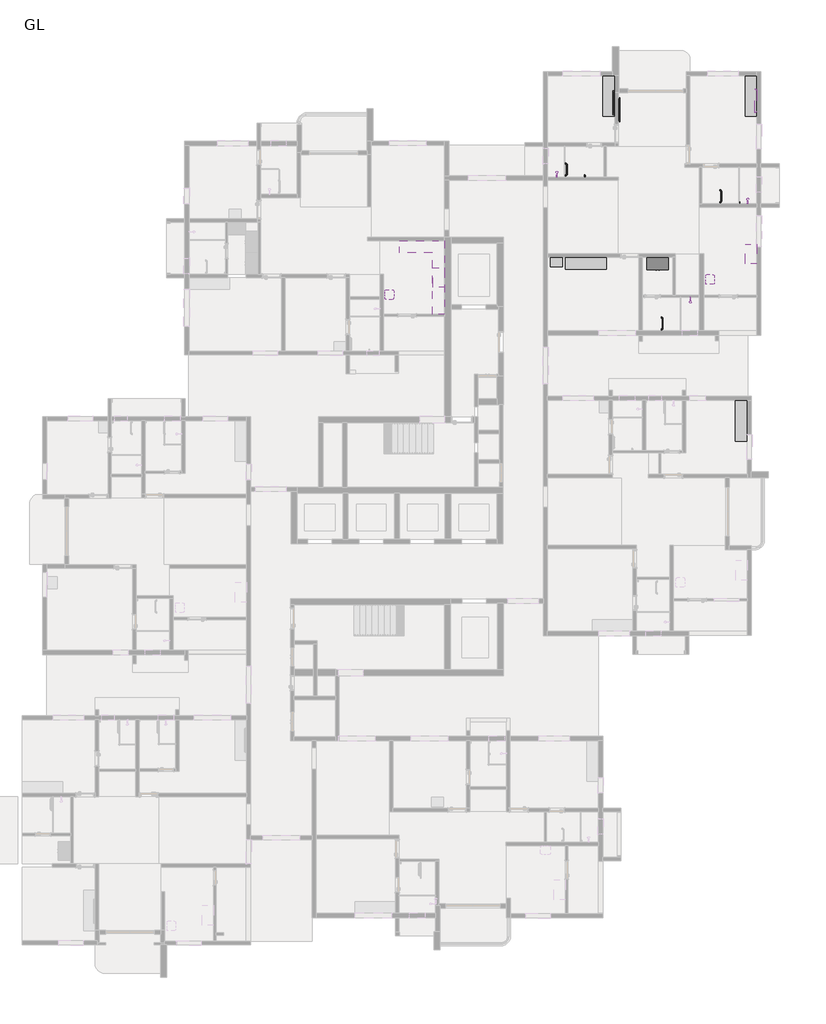
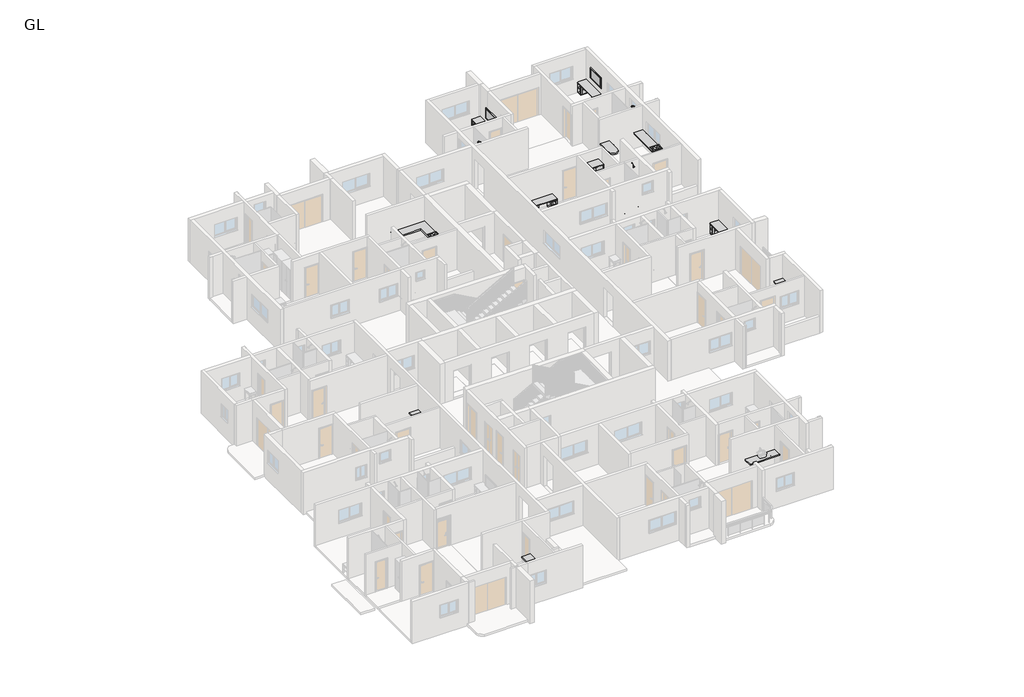
# One storey, part 14 of 14: 11 flow terminals, 9 furniture elements, 3 proxies.
"""IFC4 building model written with IfcOpenShell, lengths in millimetres."""

from ifc_helpers import new_model, si_unit, origin, place, context, project, spatial, transform, mapped, element, save
from components import cook_top_2_0915_x_500mm_892363c5, generic_models_1_generic_models_1_5b52610c, flow_terminal_f629513f, grab_rail_horizontal_grab_bar_horizontal_f73a8c0c, grab_rail_vertical_grab_rail_vertical_969059c8, plumbing_fixtures_shower_head_metal_shower_head_9404fff0, furniture_8acf2248, escritorio_de_estudiante_de_600x740mm_600_x_460_x_740mm_3f482482, furniture_eb486d47, wardrobe_family_wardrobe_large_408d0eaf

model = new_model("IFC4")

# Units and contexts
model_context = context("Model", 3, world=origin())
ifc_project = project(units=[si_unit("LENGTHUNIT", "METRE", prefix="MILLI")], contexts=[model_context])

# Site, building, storey
site = spatial("IfcSite", under=ifc_project)
building = spatial("IfcBuilding", under=site)
storey = spatial("IfcBuildingStorey", under=building, Name="GL", Elevation=0.0)

# Proxies
placement = place(None, origin())
cook_top_2_0915_x_500mm_shape = cook_top_2_0915_x_500mm_892363c5(model_context)
element("IfcBuildingElementProxy", 1, Name="Cook_Top_(2) : 0915 x 500mm", ObjectType="Cook_Top_(2) : 0915 x 500mm", at=placement, inside=storey, context=model_context, shape_type="MappedRepresentation", body=[
    mapped(cook_top_2_0915_x_500mm_shape, transform((19646.4396703, 90568.7878957, 457.2), x_axis=(0.0, 1.0, 0.0), y_axis=(-1.0, 0.0, 0.0), z_axis=(0.0, 0.0, 1.0))),
])
element("IfcBuildingElementProxy", 2, Name="Cook_Top_(2) : 0915 x 500mm", ObjectType="Cook_Top_(2) : 0915 x 500mm", at=placement, inside=storey, context=model_context, shape_type="MappedRepresentation", body=[
    mapped(cook_top_2_0915_x_500mm_shape, transform((4088.7368387, 89396.058846, 457.2), x_axis=(0.0, 1.0, 0.0), y_axis=(-1.0, 0.0, 0.0), z_axis=(0.0, 0.0, 1.0))),
])
generic_models_1_generic_models_1_shape = generic_models_1_generic_models_1_5b52610c(model_context)
element("IfcBuildingElementProxy", 3, Name="Generic Models 1 : Generic Models 1", ObjectType="Generic Models 1 : Generic Models 1", at=placement, inside=storey, context=model_context, shape_type="MappedRepresentation", body=[
    mapped(generic_models_1_generic_models_1_shape, transform((0.0, 0.0, 0.0), x_axis=(1.0, 0.0, 0.0), y_axis=(0.0, 1.0, 0.0), z_axis=(0.0, 0.0, 1.0))),
])

# Flow terminals
flow_terminal_shape = flow_terminal_f629513f(model_context)
element("IfcFlowTerminal", 4, at=placement, inside=storey, context=model_context, shape_type="MappedRepresentation", body=[
    mapped(flow_terminal_shape, transform((17568.3579642, 89283.824531, 762.0), x_axis=(0.0, 1.0, 0.0), y_axis=(-1.0, 0.0, 0.0), z_axis=(0.0, 0.0, 1.0))),
])
element("IfcFlowTerminal", 5, at=placement, inside=storey, context=model_context, shape_type="MappedRepresentation", body=[
    mapped(flow_terminal_shape, transform((1584.1551673, 88529.3280449, 762.0), x_axis=(0.0, 1.0, 0.0), y_axis=(-1.0, 0.0, 0.0), z_axis=(0.0, 0.0, 1.0))),
])
grab_rail_horizontal_grab_bar_horizontal_shape = grab_rail_horizontal_grab_bar_horizontal_f73a8c0c(model_context)
element("IfcFlowTerminal", 6, ObjectType="Grab Rail - Horizontal : Grab Bar Horizontal", at=placement, inside=storey, context=model_context, shape_type="MappedRepresentation", body=[
    mapped(grab_rail_horizontal_grab_bar_horizontal_shape, transform((10397.1569726, 93925.6073166, 0.0), x_axis=(0.0, -1.0, 0.0), y_axis=(1.0, 0.0, 0.0), z_axis=(0.0, 0.0, 1.0))),
])
element("IfcFlowTerminal", 7, ObjectType="Grab Rail - Horizontal : Grab Bar Horizontal", at=placement, inside=storey, context=model_context, shape_type="MappedRepresentation", body=[
    mapped(grab_rail_horizontal_grab_bar_horizontal_shape, transform((18099.9725595, 92589.9928672, 0.0), x_axis=(0.0, -1.0, 0.0), y_axis=(1.0, 0.0, 0.0), z_axis=(0.0, 0.0, 1.0))),
])
element("IfcFlowTerminal", 8, ObjectType="Grab Rail - Horizontal : Grab Bar Horizontal", at=placement, inside=storey, context=model_context, shape_type="MappedRepresentation", body=[
    mapped(grab_rail_horizontal_grab_bar_horizontal_shape, transform((15173.4969726, 86247.3422292, 0.0), x_axis=(0.0, -1.0, 0.0), y_axis=(1.0, 0.0, 0.0), z_axis=(0.0, 0.0, 1.0))),
])
grab_rail_vertical_grab_rail_vertical_shape = grab_rail_vertical_grab_rail_vertical_969059c8(model_context)
element("IfcFlowTerminal", 9, ObjectType="Grab Rail - Vertical : Grab Rail Vertical", at=placement, inside=storey, context=model_context, shape_type="MappedRepresentation", body=[
    mapped(grab_rail_vertical_grab_rail_vertical_shape, transform((12222.9526391, 94403.2709831, 0.0), x_axis=(1.0, 0.0, 0.0), y_axis=(0.0, 1.0, 0.0), z_axis=(0.0, 0.0, 1.0))),
])
element("IfcFlowTerminal", 10, ObjectType="Grab Rail - Vertical : Grab Rail Vertical", at=placement, inside=storey, context=model_context, shape_type="MappedRepresentation", body=[
    mapped(grab_rail_vertical_grab_rail_vertical_shape, transform((19925.768226, 93067.6565337, 0.0), x_axis=(1.0, 0.0, 0.0), y_axis=(0.0, 1.0, 0.0), z_axis=(0.0, 0.0, 1.0))),
])
element("IfcFlowTerminal", 11, ObjectType="Grab Rail - Vertical : Grab Rail Vertical", at=placement, inside=storey, context=model_context, shape_type="MappedRepresentation", body=[
    mapped(grab_rail_vertical_grab_rail_vertical_shape, transform((16999.2926391, 86744.8178957, 0.0), x_axis=(1.0, 0.0, 0.0), y_axis=(0.0, 1.0, 0.0), z_axis=(0.0, 0.0, 1.0))),
])
plumbing_fixtures_shower_head_metal_shower_head_shape = plumbing_fixtures_shower_head_metal_shower_head_9404fff0(model_context)
element("IfcFlowTerminal", 12, ObjectType="Plumbing_Fixtures_Shower_Head : Metal_Shower_Head", at=placement, inside=storey, context=model_context, shape_type="MappedRepresentation", body=[
    mapped(plumbing_fixtures_shower_head_metal_shower_head_shape, transform((9965.3569726, 94403.2709831, 1369.1616), x_axis=(1.0, 0.0, 0.0), y_axis=(0.0, 1.0, 0.0), z_axis=(0.0, 0.0, 1.0))),
])
element("IfcFlowTerminal", 13, ObjectType="Plumbing_Fixtures_Shower_Head : Metal_Shower_Head", at=placement, inside=storey, context=model_context, shape_type="MappedRepresentation", body=[
    mapped(plumbing_fixtures_shower_head_metal_shower_head_shape, transform((19477.3396703, 93067.6565337, 1369.1616), x_axis=(1.0, 0.0, 0.0), y_axis=(0.0, 1.0, 0.0), z_axis=(0.0, 0.0, 1.0))),
])
element("IfcFlowTerminal", 14, ObjectType="Plumbing_Fixtures_Shower_Head : Metal_Shower_Head", at=placement, inside=storey, context=model_context, shape_type="MappedRepresentation", body=[
    mapped(plumbing_fixtures_shower_head_metal_shower_head_shape, transform((16623.4969726, 88410.1937403, 1219.2), x_axis=(-1.0, 0.0, 0.0), y_axis=(0.0, -1.0, 0.0), z_axis=(0.0, 0.0, 1.0))),
])

# Furniture
furniture_shape = furniture_8acf2248(model_context)
element("IfcFurniture", 15, at=placement, inside=storey, context=model_context, shape_type="MappedRepresentation", body=[
    mapped(furniture_shape, transform((12853.0260982, 99452.8620895, 0.0), x_axis=(0.0, -1.0, 0.0), y_axis=(1.0, 0.0, 0.0), z_axis=(0.0, 0.0, 1.0))),
])
element("IfcFurniture", 16, at=placement, inside=storey, context=model_context, shape_type="MappedRepresentation", body=[
    mapped(furniture_shape, transform((19454.7969726, 83273.9078957, 149.9616), x_axis=(0.0, -1.0, 0.0), y_axis=(1.0, 0.0, 0.0), z_axis=(0.0, 0.0, 1.0))),
])
element("IfcFurniture", 17, at=placement, inside=storey, context=model_context, shape_type="MappedRepresentation", body=[
    mapped(furniture_shape, transform((10403.8115488, 90397.9368694, 149.9616), x_axis=(1.0, 0.0, 0.0), y_axis=(0.0, 1.0, 0.0), z_axis=(0.0, 0.0, 1.0))),
])
element("IfcFurniture", 18, at=placement, inside=storey, context=model_context, shape_type="MappedRepresentation", body=[
    mapped(furniture_shape, transform((19934.5396703, 99452.8620895, 149.9616), x_axis=(0.0, -1.0, 0.0), y_axis=(1.0, 0.0, 0.0), z_axis=(0.0, 0.0, 1.0))),
])
escritorio_de_estudiante_de_600x740mm_600_x_460_x_740mm_shape = escritorio_de_estudiante_de_600x740mm_600_x_460_x_740mm_3f482482(model_context)
element("IfcFurniture", 19, ObjectType="Escritorio_de_estudiante_de_600x740mm : 600 x 460 x 740mm", at=placement, inside=storey, context=model_context, shape_type="MappedRepresentation", body=[
    mapped(escritorio_de_estudiante_de_600x740mm_600_x_460_x_740mm_shape, transform((9946.3069726, 90169.3368694, 149.9616), x_axis=(1.0, 0.0, 0.0), y_axis=(0.0, 1.0, 0.0), z_axis=(0.0, 0.0, 1.0))),
])
furniture_2_shape = furniture_eb486d47(model_context)
element("IfcFurniture", 20, ObjectType="Furniture_TV_Plasma : 50\"", at=placement, inside=storey, context=model_context, shape_type="MappedRepresentation", body=[
    mapped(furniture_2_shape, transform((12853.0260982, 98156.1920895, 1064.3616), x_axis=(0.0, -1.0, 0.0), y_axis=(1.0, 0.0, 0.0), z_axis=(0.0, 0.0, 1.0))),
])
element("IfcFurniture", 21, ObjectType="Furniture_TV_Plasma : 50\"", at=placement, inside=storey, context=model_context, shape_type="MappedRepresentation", body=[
    mapped(furniture_2_shape, transform((13026.7620982, 97692.6420895, 0.0), x_axis=(0.0, 1.0, 0.0), y_axis=(-1.0, 0.0, 0.0), z_axis=(0.0, 0.0, 1.0))),
])
element("IfcFurniture", 22, ObjectType="Furniture_TV_Plasma : 50\"", at=placement, inside=storey, context=model_context, shape_type="MappedRepresentation", body=[
    mapped(furniture_2_shape, transform((19934.5396703, 98259.0620895, 1369.1616), x_axis=(0.0, -1.0, 0.0), y_axis=(1.0, 0.0, 0.0), z_axis=(0.0, 0.0, 1.0))),
])
wardrobe_family_wardrobe_large_shape = wardrobe_family_wardrobe_large_408d0eaf(model_context)
element("IfcFurniture", 23, ObjectType="Wardrobe-Family : Wardrobe - Large", at=placement, inside=storey, context=model_context, shape_type="MappedRepresentation", body=[
    mapped(wardrobe_family_wardrobe_large_shape, transform((14988.2069726, 90093.1368694, 149.9616), x_axis=(1.0, 0.0, 0.0), y_axis=(0.0, 1.0, 0.0), z_axis=(0.0, 0.0, 1.0))),
])

save(model, "model.ifc")

# Revit data of these elements
# Type "Cook_Top_(2) : 0915 x 500mm"
#   Keynote = "N"
#   Depth = 1.64042 ft
#   Width = 3.001969 ft
#   Material Burner = Metal - Chrome
#   Material Cooktop = Metal - Steel, Polished
#   Default Elevation = 0
# Type
#   Hauteur du plan de travail = 2.46063 ft
#   Profondeur = 1.44357 ft
#   Largeur = 1.64042 ft
#   Default Elevation = 0
# Type "Grab Rail - Horizontal : Grab Bar Horizontal"
#   Keynote = "N13"
#   Material SanitaryWare [instance default] = Metal - White powder coated
#   Default Elevation = 0
#   Assembly Code = ""
# Type "Grab Rail - Vertical : Grab Rail Vertical"
#   Keynote = "N13"
#   Material SanitaryWare [instance default] = Metal - White powder coated
#   Default Elevation = 0
#   Assembly Code = ""
# Type "Plumbing_Fixtures_Shower_Head : Metal_Shower_Head"
#   Keynote = "N13/230"
#   Mounting Height = 5.249344 ft
#   Material Shower Head = Metal - Chrome Polished
#   Default Elevation = 0
# Type
#   Default Elevation = 0
# Type "Escritorio_de_estudiante_de_600x740mm : 600 x 460 x 740mm"
#   ID_Source = "BIMTOOL"
#   ID_Objeto = "BT_F_G_836"
#   BT_Web_del_Producto = "http://www.bimtool.com/Catalog.aspx?categoria=ESCRITORIOS"
#   BT_Uso = "Interior"
#   BT_SKU = "00 00 00"
#   BT_Profundidad = "460mm"
#   BT_Peso = "N/a"
#   BT_Nombre_Técnico = "Escritorio de estudiante de 600x740mm"
#   BT_Nombre_Corto = "Escritorio de estudiante de 600x740mm"
#   BT_Material = "Madera - Acero"
#   BT_MasterFormat® = "12 00 00"
#   BT_Marca = "Bimtool"
#   BT_Itemizado_Estandar_CDT = "H 06 06 00"
#   BT_Fabricante = "Bimtool"
#   BT_Especialidad = "Mobiliario e Interiorismo"
#   BT_Elemento = "Escritorios"
#   BT_EETT = "Escritorio de estudiante de 600x740mm, con 4 apoyos de acero"
#   BT_Descripción = "Escritorio de madera"
#   BT_Código_Origen = ""
#   BT_Código_Línea = "Línea"
#   BT_Color = "N/a"
#   BT_Ancho = "600mm"
#   BT_Alto = "740mm"
#   Depth = 1.509186 ft
#   Height = 2.427822 ft
#   Width = 1.968504 ft
#   Default Elevation = 0
#   Assembly Code = ""
# Type "Furniture_TV_Plasma : 50\""
#   Keynote = "N"
#   Assembly Code = "E2020200"
#   Depth = 0.291667 ft
#   Height = 2.5 ft
#   Width = 3.958333 ft
#   Material Cabinet = Plastic - Gray
#   Default Elevation = 0
# Type "Wardrobe-Family : Wardrobe - Large"
#   Width = 2.0 ft
#   Length = 3.5 ft
#   Default Elevation = 0
# Elements 1, 2 (IfcBuildingElementProxy, "Cook_Top_(2) : 0915 x 500mm")
#   Phase Created = New Construction
#   Materials on its faces: "Metal - Chrome", "Metal - Steel, Polished"
# Element 3 (IfcBuildingElementProxy, "Generic Models 1 : Generic Models 1")
#   Phase Created = New Construction
#   Materials on its faces: "HALL"
# Elements 4, 5 (IfcFlowTerminal)
#   Phase Created = New Construction
# Elements 6, 7, 8 (IfcFlowTerminal, "Grab Rail - Horizontal : Grab Bar Horizontal")
#   Material SanitaryWare = Metal - White powder coated
#   Phase Created = New Construction
#   Materials on its faces: "Metal - White powder coated"
# Elements 9, 10, 11 (IfcFlowTerminal, "Grab Rail - Vertical : Grab Rail Vertical")
#   Material SanitaryWare = Metal - White powder coated
#   Phase Created = New Construction
#   Materials on its faces: "Metal - White powder coated"
# Elements 12, 13, 14 (IfcFlowTerminal, "Plumbing_Fixtures_Shower_Head : Metal_Shower_Head")
#   Phase Created = New Construction
#   Materials on its faces: "Metal - Chrome Polished"
# Elements 15, 16, 17, 18 (IfcFurniture)
#   Phase Created = New Construction
# Element 19 (IfcFurniture, "Escritorio_de_estudiante_de_600x740mm : 600 x 460 x 740mm")
#   Phase Created = New Construction
#   Materials on its faces: "Metal - Chrome", "Wood - Birch", "Metal - Steel"
# Elements 20, 21, 22 (IfcFurniture, "Furniture_TV_Plasma : 50\"")
#   Phase Created = New Construction
#   Materials on its faces: "Plastic - Black", "Plastic - Gray", "Glass"
# Element 23 (IfcFurniture, "Wardrobe-Family : Wardrobe - Large")
#   Phase Created = New Construction
#   Materials on its faces: "Wood Material", "Steel Handle"
# Materials
#   "Metal - Chrome": colour RGB 247 247 247, transparency 0
#   "Metal - Steel, Polished": colour RGB 247 247 247, transparency 0
#   "Metal - White powder coated": colour RGB 249 249 249, transparency 0
#   "Metal - Chrome Polished": colour RGB 247 247 247, transparency 0
#   "Plastic - Gray": class "Plastic", colour RGB 134 134 134, transparency 0
#   "HALL": class "Generic", colour RGB 120 120 120, transparency 0, Cost = 0
#   "Wood - Birch": class "Wood", colour RGB 213 164 103, transparency 0
#   "Metal - Steel": colour RGB 247 247 247, transparency 0
#   "Plastic - Black": colour RGB 0 0 0, transparency 0
#   "Glass": class "Glass", colour RGB 0 128 192, transparency 0.9, Description = "Soda Lime Glass", Cost = 0
#   "Wood Material": class "Generic", colour RGB 128 72 40, transparency 0, Cost = 0
#   "Steel Handle": class "Generic", colour RGB 206 211 212, transparency 0, Cost = 0
